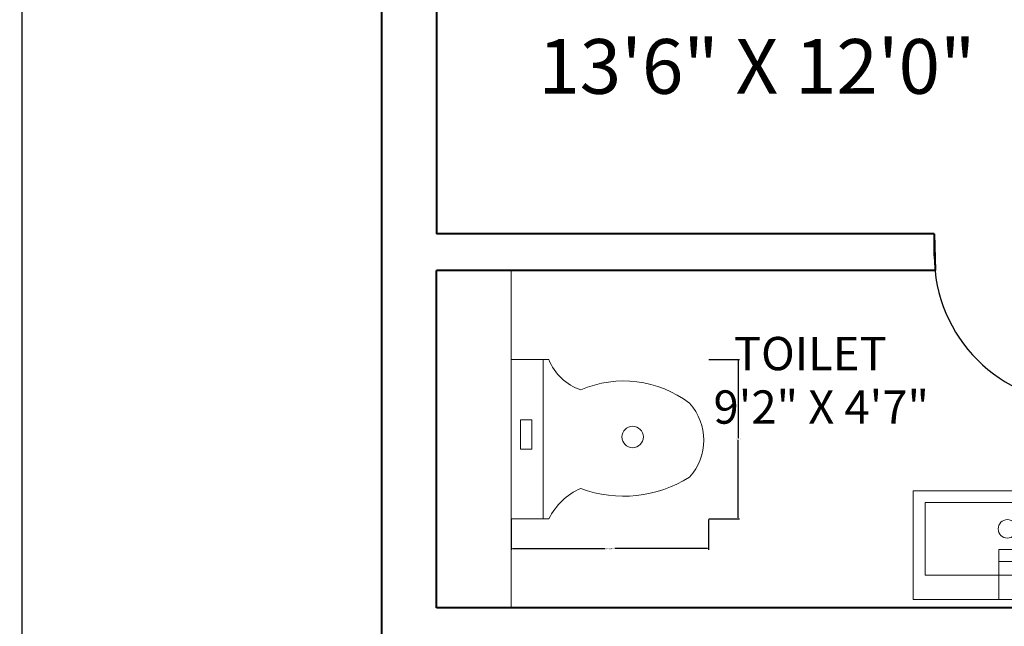
# Model space of a CAD drawing. Units: inches. Extents: x -46 to 1145, y -527 to 760.
# Tile 34 of 57: x -46 to 114, y 443 to 541. Entities that reach past the tile are written whole.
import ezdxf

# ---------------------------------------------------------------- set-up
doc = ezdxf.new("R2010")
doc.units = ezdxf.units.IN
doc.header["$MEASUREMENT"] = 0
for name, color, linetype, lineweight in [('A-ANNO-DIMS', 2, 'Continuous', 18), ('A-AREA-IDEN', 1, 'Continuous', 18), ('A-FLOR-CASE', 32, 'Continuous', 18), ('A-FLOR-FIXT', 9, 'Continuous', 18), ('DOORS', 3, 'Continuous', 25), ('WALLS', 4, 'Continuous', 40)]:
    doc.layers.add(name, color=color, linetype=linetype, lineweight=lineweight)
doc.styles.get("Standard").update_dxf_attribs({"font": 'arial.ttf'})
doc.dimstyles.get("Standard").update_dxf_attribs({"dimtxt": 0.18, "dimasz": 0.18, "dimexe": 0.18, "dimexo": 0.0625, "dimgap": 0.09, "dimtad": 0, "dimtih": 1, "dimtoh": 1, "dimdec": 0, "dimzin": 0, "dimdsep": 46, "dimlunit": 3, "dimtxsty": 'Standard', "dimcen": 0.09, "dimadec": 0, "dimazin": 0, "dimtfac": 1, "dimtdec": 0, "dimtofl": 0, "dimtmove": 0, "dimatfit": 3, "dimfxl": 1, "dimtolj": 1, "dimtzin": 0, "dimarcsym": 0})

# ---------------------------------------------------------------- blocks, each defined once
blk = doc.blocks.new('*U2')
for p, q in [((0, 0), (0, -6)), ((40, 0), (40, -6))]:
    blk.add_line(p, q)
blk.add_lwpolyline([(0, 0), (0, 40), (1.75, 40), (1.75, 0)], close=True)
blk.add_arc((0, 0), 40, 0, 90)
blk = doc.blocks.new('LAVATORY-RECT')
blk.add_line((14.01, 6.17), (17.08, 6.17))
for points in [[(30.61, 0), (0, 0), (0, 17.7), (30.61, 17.7)], [(28.7, 3.94), (1.97, 3.94), (1.97, 15.81), (28.7, 15.81)], [(17.08, 0), (14.01, 0), (14.01, 8.17), (17.08, 8.17)]]:
    blk.add_lwpolyline(points, close=True)
blk.add_circle((15.39, 11.51), 1.51)
blk = doc.blocks.new('WATER-CLOSET')
for p, q in [((0, 0), (0, 26.01)), ((0, 26.01), (6.13, 26.01)), ((5.22, 21.04), (5.22, 26.01)), ((5.22, 26.01), (5.22, 0)), ((0, 0), (6.13, 0))]:
    blk.add_line(p, q)
blk.add_lwpolyline([(1.51, 11.4), (1.51, 16.16), (3.34, 16.16), (3.34, 11.4)], close=True)
blk.add_circle((19.79, 13.37), 1.75)
for centre, radius, start, end in [((14.15, 29.2), 8.64, 201.6782, 251.0259), ((18.35, 4.96), 17.54, 52.4616, 113.5359), ((22.52, 12.84), 8.87, 317.2682, 42.7318), ((18.33, 23.71), 20, 249.5645, 302.3709), ((15.4, -4.5), 10.31, 113.1704, 154.0947)]:
    blk.add_arc(centre, radius, start, end)
blk = doc.blocks.new('*D660')
at = {"layer": 'A-ANNO-DIMS', "color": 0, "lineweight": -2, "transparency": 16777216}
for p, q in [((33.74, 459.95), (33.74, 455)), ((65.92, 459.95), (65.92, 455)), ((33.92, 455.18), (49.06, 455.18)), ((65.74, 455.18), (50.61, 455.18))]:
    blk.add_line(p, q, dxfattribs=at)
at = {"layer": 'A-ANNO-DIMS', "color": 0, "transparency": 16777216}
for points in [[(33.92, 455.21), (33.92, 455.15), (33.74, 455.18)], [(65.74, 455.21), (65.74, 455.15), (65.92, 455.18)]]:
    blk.add_solid(points, dxfattribs=at)
at = {"layer": 'Defpoints', "color": 0, "transparency": 16777216}
for p in [(33.74, 460.01), (65.92, 460.01), (65.92, 455.18)]:
    blk.add_point(p, dxfattribs=at)
at = {"layer": 'A-ANNO-DIMS', "color": 0, "transparency": 16777216, "insert": (49.83, 455.18), "char_height": 0.18, "attachment_point": 5}
blk.add_mtext('\\A1;WC 32 TYP.', dxfattribs=at)
blk = doc.blocks.new('*D661')
at = {"layer": 'A-ANNO-DIMS', "color": 0, "lineweight": -2, "transparency": 16777216}
for p, q in [((65.98, 486.02), (70.93, 486.02)), ((70.75, 485.84), (70.75, 473.2)), ((70.75, 460.19), (70.75, 472.84)), ((65.98, 460.01), (70.93, 460.01))]:
    blk.add_line(p, q, dxfattribs=at)
at = {"layer": 'A-ANNO-DIMS', "color": 0, "transparency": 16777216}
for points in [[(70.72, 485.84), (70.78, 485.84), (70.75, 486.02)], [(70.72, 460.19), (70.78, 460.19), (70.75, 460.01)]]:
    blk.add_solid(points, dxfattribs=at)
at = {"layer": 'Defpoints', "color": 0, "transparency": 16777216}
for p in [(65.92, 486.02), (70.75, 486.02), (65.92, 460.01)]:
    blk.add_point(p, dxfattribs=at)
at = {"layer": 'A-ANNO-DIMS', "color": 0, "transparency": 16777216, "insert": (70.75, 473.02), "char_height": 0.18, "attachment_point": 5}
blk.add_mtext('\\A1;26 TYP.', dxfattribs=at)
blk = doc.blocks.new('*D685')
at = {"layer": 'A-ANNO-DIMS', "color": 0, "lineweight": -2, "transparency": 16777216}
for p, q in [((183.5, 700.89), (-46.22, 700.89)), ((-46.04, 700.71), (-46.04, 116.39)), ((-46.04, -468.3), (-46.04, 116.02)), ((12.5, -468.48), (-46.22, -468.48))]:
    blk.add_line(p, q, dxfattribs=at)
at = {"layer": 'A-ANNO-DIMS', "color": 0, "transparency": 16777216}
for points in [[(-46.07, 700.71), (-46.01, 700.71), (-46.04, 700.89)], [(-46.07, -468.3), (-46.01, -468.3), (-46.04, -468.48)]]:
    blk.add_solid(points, dxfattribs=at)
at = {"layer": 'Defpoints', "color": 0, "transparency": 16777216}
for p in [(-46.04, 700.89), (183.56, 700.89), (12.56, -468.48)]:
    blk.add_point(p, dxfattribs=at)
at = {"layer": 'A-ANNO-DIMS', "color": 0, "transparency": 16777216, "insert": (-46.04, 116.2), "char_height": 0.18, "attachment_point": 5}
blk.add_mtext('\\A1;1169.4', dxfattribs=at)

msp = doc.modelspace()

# ---------------------------------------------------------------- linework, layer by layer
at = {"layer": 'A-FLOR-CASE'}
msp.add_line((33.7427, 500.5176), (33.7427, 445.5176), dxfattribs=at)
at = {"layer": 'WALLS'}
for p, q in [((12.5637, 659.5176), (12.5637, 221.5176)), ((21.5637, 650.5176), (21.5637, 506.5176)), ((102.7169, 506.5176), (21.5637, 506.5176)), ((102.7169, 506.5176), (102.8372, 500.5176)), ((21.5637, 445.5176), (21.5637, 500.5176)), ((102.8372, 500.5176), (21.5637, 500.5176)), ((131.5637, 445.5176), (21.5637, 445.5176))]:
    msp.add_line(p, q, dxfattribs=at)

# ---------------------------------------------------------------- block references
at = {"layer": 'A-FLOR-FIXT'}
for name, p in [('WATER-CLOSET', (33.743, 460.011)), ('LAVATORY-RECT', (99.252, 446.889))]:
    msp.add_blockref(name, p, dxfattribs=at)
at = {"layer": 'DOORS', "xscale": 0.6, "yscale": 0.6, "zscale": 0.6, "rotation": 180}
msp.add_blockref('*U2', (126.7169, 502.9176), dxfattribs=at)

# ---------------------------------------------------------------- texts
at = {"layer": 'A-AREA-IDEN'}
for s, height, p in [('13\'6" X 12\'0"', 8.923264, (38.1454, 529.3164)), ('   TOILET', 5.42821, (65.0585, 484.264)), (' 9\'2" X 4\'7"', 5.428214, (65.0585, 475.544))]:
    msp.add_text(s, height=height, dxfattribs=at).set_placement(p)

# ---------------------------------------------------------------- dimensions: what is measured, and where the dimension line sits
at = {"layer": 'A-ANNO-DIMS'}
dim = msp.add_linear_dim(base=(-46.0363, 700.8886), p1=(12.5637, -468.4824), p2=(183.5637, 700.8886), angle=90, dimstyle='Standard', override={"dimdec": 1, "dimlfac": 1, "dimrnd": 0, "dimzin": 0, "dimdsep": 46, "dimlunit": 2}, dxfattribs=at)
dim.commit()
dim.dimension.update_dxf_attribs({"geometry": '*D685', "text_midpoint": (-46.0363, 116.2031)})
dim = msp.add_linear_dim(base=(70.7473, 486.0244), p1=(65.9206, 460.0108), p2=(65.9206, 486.0244), angle=90, text='<> TYP.', dimstyle='Standard', override={"dimdec": 0, "dimlfac": 1, "dimrnd": 0, "dimzin": 0, "dimdsep": 46, "dimlunit": 2}, dxfattribs=at)
dim.commit()
dim.dimension.update_dxf_attribs({"geometry": '*D661', "text_midpoint": (70.7473, 473.0176)})
dim = msp.add_linear_dim(base=(65.9206, 455.1841), p1=(33.7427, 460.0108), p2=(65.9206, 460.0108), text='WC <> TYP.', dimstyle='Standard', override={"dimdec": 0, "dimlfac": 1, "dimrnd": 0, "dimzin": 0, "dimdsep": 46, "dimlunit": 2}, dxfattribs=at)
dim.commit()
dim.dimension.update_dxf_attribs({"geometry": '*D660', "text_midpoint": (49.8316, 455.1841)})

doc.saveas('drawing.dxf')
